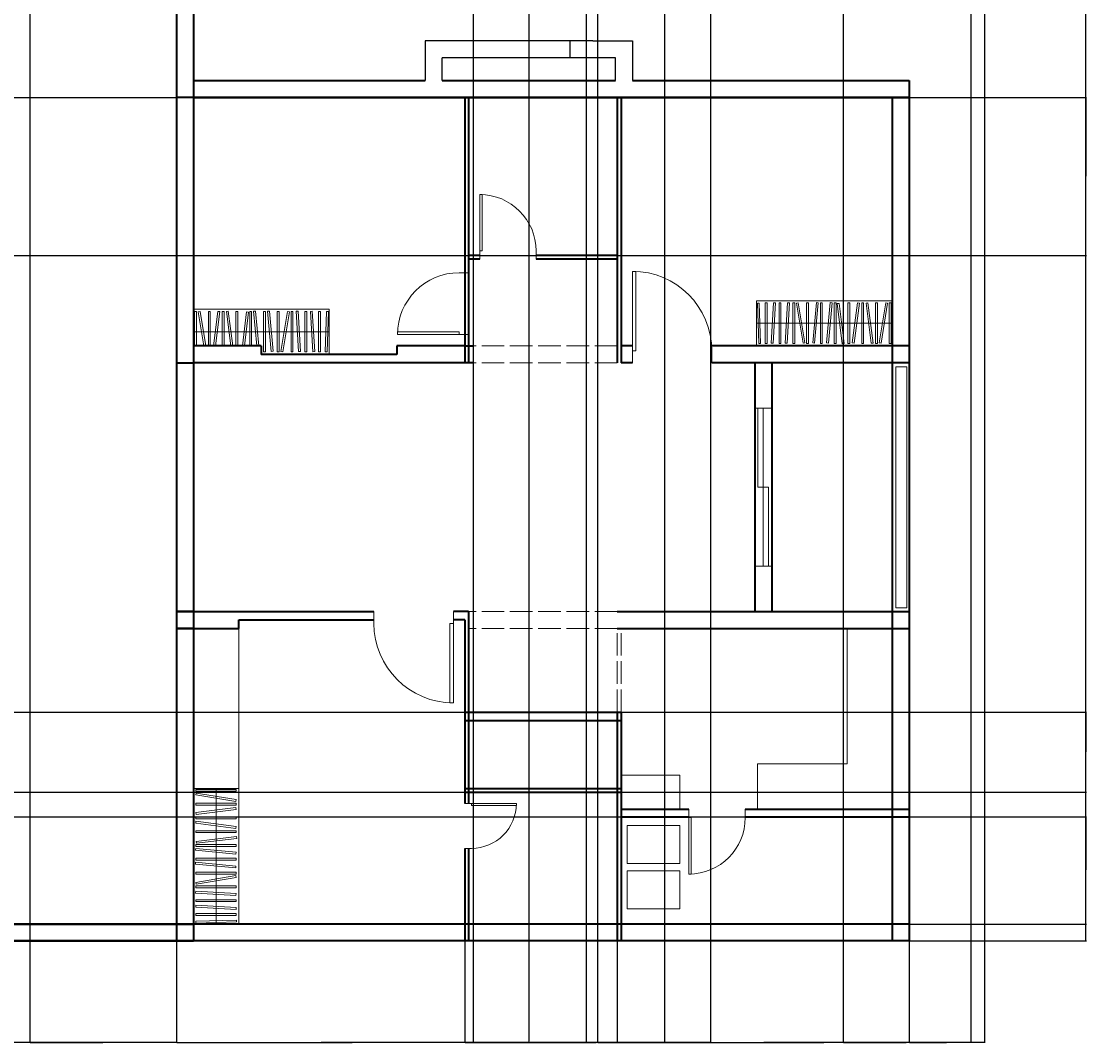
# Model space of a CAD drawing. Units: inches. Extents: x 531915 to 533151, y 849859 to 851471.
# Tile 4 of 7: x 532585 to 533151, y 850315 to 850858. Entities that reach past the tile are written whole.
import ezdxf

# ---------------------------------------------------------------- set-up
doc = ezdxf.new("R2010")
doc.units = ezdxf.units.IN
doc.linetypes.add('ACAD_ISO02W100', pattern=[15, 12, -3])
for name, color, linetype, lineweight in [('A-ANNO-DIMS', 2, 'Continuous', 18), ('A-DOOR', 3, 'Continuous', 18), ('A-FLOR-CASE', 9, 'Continuous', 18), ('A-FLOR-FIXT', 8, 'Continuous', 18), ('A-FLOR-HRAL', 4, 'Continuous', 20), ('A-FLOR-SLAB', 7, 'Continuous', 25), ('A-FURN', 8, 'Continuous', 13), ('A-NPLT-CNST', 9, 'Continuous', 9), ('A-WALL', 7, 'Continuous', 35), ('A-WALL-OVHD', 7, 'ACAD_ISO02W100', 18)]:
    doc.layers.add(name, color=color, linetype=linetype, lineweight=lineweight)
doc.styles.get("Standard").update_dxf_attribs({"font": 'arial.ttf'})
doc.dimstyles.get("Standard").update_dxf_attribs({"dimtxt": 0.18, "dimasz": 0.18, "dimexe": 0.18, "dimexo": 0.0625, "dimgap": 0.09, "dimtad": 0, "dimtih": 1, "dimtoh": 1, "dimdec": 4, "dimzin": 0, "dimdsep": 46, "dimtxsty": 'Standard', "dimcen": 0.09, "dimadec": 0, "dimazin": 0, "dimtfac": 1, "dimtdec": 4, "dimtofl": 0, "dimtmove": 0, "dimatfit": 3, "dimfxl": 1, "dimtolj": 1, "dimtzin": 0, "dimarcsym": 0})

# ---------------------------------------------------------------- blocks, each defined once
blk = doc.blocks.new('*U2')
for p, q in [((0, 0), (0, -6)), ((40, 0), (40, -6))]:
    blk.add_line(p, q)
blk.add_lwpolyline([(0, 0), (0, 40), (1.75, 40), (1.75, 0)], close=True)
blk.add_arc((0, 0), 40, 0, 90)
blk = doc.blocks.new('WARDROBE-72')
blk.add_line((12, 0), (12, 72))
for points in [[(24, 0), (24, 72), (0, 72), (0, 0)], [(1.15, 70.47), (1.15, 71.48), (22.64, 71.48), (22.64, 70.47)], [(1.21, 68.56), (1.37, 69.55), (22.58, 66.07), (22.41, 65.07)], [(1.15, 63.15), (1.15, 64.16), (22.64, 64.16), (22.64, 63.15)], [(1.15, 55.83), (1.15, 56.84), (22.64, 56.84), (22.64, 55.83)], [(1.3, 58.13), (1.17, 59.13), (22.48, 61.86), (22.61, 60.86)], [(1.11, 53.59), (1.24, 54.59), (22.54, 51.79), (22.41, 50.79)], [(1.15, 48.51), (1.15, 49.52), (22.64, 49.52), (22.64, 48.51)], [(1.55, 42.84), (1.42, 43.84), (22.76, 46.42), (22.88, 45.42)], [(1.04, 39.13), (1.13, 40.14), (22.52, 38.16), (22.43, 37.15)], [(1.15, 41.19), (1.15, 42.2), (22.64, 42.2), (22.64, 41.19)], [(1.15, 33.87), (1.15, 34.88), (22.64, 34.88), (22.64, 33.87)], [(0.98, 31.76), (1.07, 32.76), (22.47, 30.78), (22.37, 29.78)], [(1.15, 26.55), (1.15, 27.56), (22.64, 27.56), (22.64, 26.55)], [(1.38, 21.1), (1.21, 22.1), (22.4, 25.68), (22.57, 24.68)], [(1.05, 16.46), (1.11, 17.47), (22.56, 16.21), (22.5, 15.2)], [(1.15, 19.23), (1.15, 20.24), (22.64, 20.24), (22.64, 19.23)], [(1.15, 11.91), (1.15, 12.92), (22.64, 12.92), (22.64, 11.91)], [(1.11, 8.97), (1.17, 9.98), (22.62, 8.71), (22.56, 7.7)], [(1.15, 4.59), (1.15, 5.6), (22.64, 5.6), (22.64, 4.59)], [(1.25, 0.42), (1.22, 1.43), (22.7, 2.11), (22.73, 1.1)]]:
    blk.add_lwpolyline(points, close=True)
blk = doc.blocks.new('WARDROBE-72-RECESSED')
blk.add_line((0, 12), (72, 12))
for points in [[(72, 0), (72, 24), (0, 24), (0, 0), (36.16, 0)], [(37.42, 4.5), (39.13, 22.96), (40.14, 22.87), (38.44, 4.5)], [(41.19, 4.5), (41.19, 22.85), (42.2, 22.85), (42.2, 4.5)], [(48.51, 4.5), (48.51, 22.85), (49.52, 22.85), (49.52, 4.5)], [(51.17, 4.5), (53.59, 22.89), (54.59, 22.76), (52.19, 4.5)], [(55.83, 4.5), (55.83, 22.85), (56.84, 22.85), (56.84, 4.5)], [(60.46, 4.5), (58.13, 22.7), (59.13, 22.83), (61.48, 4.5)], [(63.15, 4.5), (63.15, 22.85), (64.16, 22.85), (64.16, 4.5)], [(65.55, 4.5), (68.56, 22.79), (69.55, 22.63), (66.57, 4.5)], [(70.47, 4.5), (70.47, 22.85), (71.48, 22.85), (71.48, 4.5)], [(45.01, 4.5), (42.84, 22.45), (43.84, 22.58), (46.03, 4.5)]]:
    blk.add_lwpolyline(points)
for points in [[(0.42, 22.75), (1.43, 22.78), (2.11, 1.3), (1.1, 1.27)], [(4.59, 22.85), (5.6, 22.85), (5.6, 1.36), (4.59, 1.36)], [(8.97, 22.89), (9.98, 22.83), (8.71, 1.38), (7.7, 1.44)], [(11.91, 22.85), (12.92, 22.85), (12.92, 1.36), (11.91, 1.36)], [(16.46, 22.95), (17.47, 22.89), (16.21, 1.44), (15.2, 1.5)], [(19.23, 22.85), (20.24, 22.85), (20.24, 1.36), (19.23, 1.36)], [(21.1, 22.62), (22.1, 22.79), (25.68, 1.6), (24.68, 1.43)], [(26.55, 22.85), (27.56, 22.85), (27.56, 1.36), (26.55, 1.36)], [(31.76, 23.02), (32.76, 22.93), (30.78, 1.53), (29.78, 1.63)], [(33.87, 22.85), (34.88, 22.85), (34.88, 1.36), (33.87, 1.36)]]:
    blk.add_lwpolyline(points, close=True)
blk = doc.blocks.new('BALCONY-SLIDER-84')
blk.add_line((2.88, 84), (2.88, 0))
for points in [[(2.88, 84), (5.76, 84), (5.76, 41.94), (2.88, 41.94)], [(2.88, 41.94), (0, 41.94), (0, 0), (2.88, 0)]]:
    blk.add_lwpolyline(points, close=True)
blk = doc.blocks.new('UTILITY-FIXTURES-PAIR')
for points in [[(0, 24.11), (28.12, 24.11), (28.12, 44.31), (0, 44.31)], [(0, 0), (28.12, 0), (28.12, 20.2), (0, 20.2)]]:
    blk.add_lwpolyline(points, close=True)
blk = doc.blocks.new('SERVICE-LEDGE-110')
for p, q in [((21, 21), (0, 21)), ((0, 21), (0, 0)), ((21, 21), (101, 21)), ((33, 12), (33, 21)), ((101, 21), (110, 21)), ((110, 21), (110, 0)), ((9, 0), (9, 12)), ((9, 12), (21, 12)), ((9, 12), (33, 12)), ((21, 12), (101, 12)), ((101, 0), (101, 12))]:
    blk.add_line(p, q)
blk = doc.blocks.new('COUNTER-L-RETURN')
for p, q in [((47.51, 96), (47.51, 24)), ((0, 24), (47.51, 24)), ((0, 24), (0, 0))]:
    blk.add_line(p, q)
blk = doc.blocks.new('COUNTER-END-RETURN')
for p in [(0, 18), (31.29, 0)]:
    blk.add_line(p, (31.29, 18))
blk = doc.blocks.new('*D38')
at = {"layer": 'A-ANNO-DIMS', "color": 0, "lineweight": -2, "transparency": 16777216}
for p, q in [((533096.87, 851416.87), (533150.9, 851416.87)), ((533150.72, 851416.69), (533150.72, 850893.31)), ((533150.72, 850369.55), (533150.72, 850892.94)), ((533056.87, 850369.37), (533150.9, 850369.37))]:
    blk.add_line(p, q, dxfattribs=at)
at = {"layer": 'A-ANNO-DIMS', "color": 0, "transparency": 16777216}
for points in [[(533150.69, 851416.69), (533150.75, 851416.69), (533150.72, 851416.87)], [(533150.69, 850369.55), (533150.75, 850369.55), (533150.72, 850369.37)]]:
    blk.add_solid(points, dxfattribs=at)
at = {"layer": 'Defpoints', "color": 0, "transparency": 16777216}
for p in [(533096.8, 851416.87), (533056.8, 850369.37), (533150.72, 850369.37)]:
    blk.add_point(p, dxfattribs=at)
at = {"layer": 'A-ANNO-DIMS', "color": 0, "transparency": 16777216, "insert": (533150.72, 850893.12), "char_height": 0.18, "attachment_point": 5}
blk.add_mtext('\\A1;1047.5', dxfattribs=at)
blk = doc.blocks.new('*D42')
at = {"layer": 'A-ANNO-DIMS', "color": 0, "lineweight": -2, "transparency": 16777216}
for p, q in [((532451.8, 850369.31), (532451.8, 850315.34)), ((532667.8, 850369.31), (532667.8, 850315.34)), ((532451.98, 850315.52), (532559.51, 850315.52)), ((532667.62, 850315.52), (532560.1, 850315.52))]:
    blk.add_line(p, q, dxfattribs=at)
at = {"layer": 'A-ANNO-DIMS', "color": 0, "transparency": 16777216}
for points in [[(532451.98, 850315.55), (532451.98, 850315.49), (532451.8, 850315.52)], [(532667.62, 850315.55), (532667.62, 850315.49), (532667.8, 850315.52)]]:
    blk.add_solid(points, dxfattribs=at)
at = {"layer": 'Defpoints', "color": 0, "transparency": 16777216}
for p in [(532451.8, 850369.37), (532667.8, 850369.37), (532667.8, 850315.52)]:
    blk.add_point(p, dxfattribs=at)
at = {"layer": 'A-ANNO-DIMS', "color": 0, "transparency": 16777216, "insert": (532559.8, 850315.52), "char_height": 0.18, "attachment_point": 5}
blk.add_mtext('\\A1;216', dxfattribs=at)
blk = doc.blocks.new('*D43')
at = {"layer": 'A-ANNO-DIMS', "color": 0, "lineweight": -2, "transparency": 16777216}
for p, q in [((532667.8, 850369.31), (532667.8, 850315.34)), ((532820.8, 850369.31), (532820.8, 850315.34)), ((532667.98, 850315.52), (532744.02, 850315.52)), ((532820.62, 850315.52), (532744.59, 850315.52))]:
    blk.add_line(p, q, dxfattribs=at)
at = {"layer": 'A-ANNO-DIMS', "color": 0, "transparency": 16777216}
for points in [[(532667.98, 850315.55), (532667.98, 850315.49), (532667.8, 850315.52)], [(532820.62, 850315.55), (532820.62, 850315.49), (532820.8, 850315.52)]]:
    blk.add_solid(points, dxfattribs=at)
at = {"layer": 'Defpoints', "color": 0, "transparency": 16777216}
for p in [(532667.8, 850369.37), (532820.8, 850369.37), (532820.8, 850315.52)]:
    blk.add_point(p, dxfattribs=at)
at = {"layer": 'A-ANNO-DIMS', "color": 0, "transparency": 16777216, "insert": (532744.3, 850315.52), "char_height": 0.18, "attachment_point": 5}
blk.add_mtext('\\A1;153', dxfattribs=at)
blk = doc.blocks.new('*D44')
at = {"layer": 'A-ANNO-DIMS', "color": 0, "lineweight": -2, "transparency": 16777216}
for p, q in [((532820.8, 850369.31), (532820.8, 850315.34)), ((532901.8, 850369.31), (532901.8, 850315.34)), ((532820.98, 850315.52), (532861.1, 850315.52)), ((532901.62, 850315.52), (532861.51, 850315.52))]:
    blk.add_line(p, q, dxfattribs=at)
at = {"layer": 'A-ANNO-DIMS', "color": 0, "transparency": 16777216}
for points in [[(532820.98, 850315.55), (532820.98, 850315.49), (532820.8, 850315.52)], [(532901.62, 850315.55), (532901.62, 850315.49), (532901.8, 850315.52)]]:
    blk.add_solid(points, dxfattribs=at)
at = {"layer": 'Defpoints', "color": 0, "transparency": 16777216}
for p in [(532820.8, 850369.37), (532901.8, 850369.37), (532901.8, 850315.52)]:
    blk.add_point(p, dxfattribs=at)
at = {"layer": 'A-ANNO-DIMS', "color": 0, "transparency": 16777216, "insert": (532861.3, 850315.52), "char_height": 0.18, "attachment_point": 5}
blk.add_mtext('\\A1;81', dxfattribs=at)
blk = doc.blocks.new('*D45')
at = {"layer": 'A-ANNO-DIMS', "color": 0, "lineweight": -2, "transparency": 16777216}
for p, q in [((532901.8, 850369.31), (532901.8, 850315.34)), ((533056.8, 850369.31), (533056.8, 850315.34)), ((532901.98, 850315.52), (532979.02, 850315.52)), ((533056.62, 850315.52), (532979.59, 850315.52))]:
    blk.add_line(p, q, dxfattribs=at)
at = {"layer": 'A-ANNO-DIMS', "color": 0, "transparency": 16777216}
for points in [[(532901.98, 850315.55), (532901.98, 850315.49), (532901.8, 850315.52)], [(533056.62, 850315.55), (533056.62, 850315.49), (533056.8, 850315.52)]]:
    blk.add_solid(points, dxfattribs=at)
at = {"layer": 'Defpoints', "color": 0, "transparency": 16777216}
for p in [(532901.8, 850369.37), (533056.8, 850369.37), (533056.8, 850315.52)]:
    blk.add_point(p, dxfattribs=at)
at = {"layer": 'A-ANNO-DIMS', "color": 0, "transparency": 16777216, "insert": (532979.3, 850315.52), "char_height": 0.18, "attachment_point": 5}
blk.add_mtext('\\A1;155', dxfattribs=at)
blk = doc.blocks.new('*D47')
at = {"layer": 'A-ANNO-DIMS', "color": 0, "lineweight": -2, "transparency": 16777216}
for p, q in [((533096.8, 850946.31), (533096.8, 850315.34)), ((533056.8, 850826.31), (533056.8, 850315.34)), ((533056.98, 850315.52), (533076.58, 850315.52)), ((533096.62, 850315.52), (533077.03, 850315.52))]:
    blk.add_line(p, q, dxfattribs=at)
at = {"layer": 'A-ANNO-DIMS', "color": 0, "transparency": 16777216}
for points in [[(533056.98, 850315.55), (533056.98, 850315.49), (533056.8, 850315.52)], [(533096.62, 850315.55), (533096.62, 850315.49), (533096.8, 850315.52)]]:
    blk.add_solid(points, dxfattribs=at)
at = {"layer": 'Defpoints', "color": 0, "transparency": 16777216}
for p in [(533096.8, 850946.37), (533056.8, 850826.37), (533056.8, 850315.52)]:
    blk.add_point(p, dxfattribs=at)
at = {"layer": 'A-ANNO-DIMS', "color": 0, "transparency": 16777216, "insert": (533076.8, 850315.52), "char_height": 0.18, "attachment_point": 5}
blk.add_mtext('\\A1;40', dxfattribs=at)
blk = doc.blocks.new('*D49')
at = {"layer": 'A-ANNO-DIMS', "color": 0, "lineweight": -2, "transparency": 16777216}
for p, q in [((532825.3, 851312.76), (532825.3, 850315.34)), ((532885.3, 851312.76), (532885.3, 850315.34)), ((532825.48, 850315.52), (532855.09, 850315.52)), ((532885.12, 850315.52), (532855.52, 850315.52))]:
    blk.add_line(p, q, dxfattribs=at)
at = {"layer": 'A-ANNO-DIMS', "color": 0, "transparency": 16777216}
for points in [[(532825.48, 850315.55), (532825.48, 850315.49), (532825.3, 850315.52)], [(532885.12, 850315.55), (532885.12, 850315.49), (532885.3, 850315.52)]]:
    blk.add_solid(points, dxfattribs=at)
at = {"layer": 'Defpoints', "color": 0, "transparency": 16777216}
for p in [(532825.3, 851312.82), (532885.3, 851312.82), (532885.3, 850315.52)]:
    blk.add_point(p, dxfattribs=at)
at = {"layer": 'A-ANNO-DIMS', "color": 0, "transparency": 16777216, "insert": (532855.3, 850315.52), "char_height": 0.18, "attachment_point": 5}
blk.add_mtext('\\A1;60', dxfattribs=at)
blk = doc.blocks.new('*D50')
at = {"layer": 'A-ANNO-DIMS', "color": 0, "lineweight": -2, "transparency": 16777216}
for p, q in [((532891.3, 851312.76), (532891.3, 850315.34)), ((532951.3, 851312.76), (532951.3, 850315.34)), ((532891.48, 850315.52), (532921.09, 850315.52)), ((532951.12, 850315.52), (532921.52, 850315.52))]:
    blk.add_line(p, q, dxfattribs=at)
at = {"layer": 'A-ANNO-DIMS', "color": 0, "transparency": 16777216}
for points in [[(532891.48, 850315.55), (532891.48, 850315.49), (532891.3, 850315.52)], [(532951.12, 850315.55), (532951.12, 850315.49), (532951.3, 850315.52)]]:
    blk.add_solid(points, dxfattribs=at)
at = {"layer": 'Defpoints', "color": 0, "transparency": 16777216}
for p in [(532891.3, 851312.82), (532951.3, 851312.82), (532951.3, 850315.52)]:
    blk.add_point(p, dxfattribs=at)
at = {"layer": 'A-ANNO-DIMS', "color": 0, "transparency": 16777216, "insert": (532921.3, 850315.52), "char_height": 0.18, "attachment_point": 5}
blk.add_mtext('\\A1;60', dxfattribs=at)
blk = doc.blocks.new('*D55')
at = {"layer": 'A-ANNO-DIMS', "color": 0, "lineweight": -2, "transparency": 16777216}
for p, q in [((532667.8, 850946.31), (532667.8, 850315.34)), ((532854.8, 850946.31), (532854.8, 850315.34)), ((532667.98, 850315.52), (532761.02, 850315.52)), ((532854.62, 850315.52), (532761.59, 850315.52))]:
    blk.add_line(p, q, dxfattribs=at)
at = {"layer": 'A-ANNO-DIMS', "color": 0, "transparency": 16777216}
for points in [[(532667.98, 850315.55), (532667.98, 850315.49), (532667.8, 850315.52)], [(532854.62, 850315.55), (532854.62, 850315.49), (532854.8, 850315.52)]]:
    blk.add_solid(points, dxfattribs=at)
at = {"layer": 'Defpoints', "color": 0, "transparency": 16777216}
for p in [(532667.8, 850946.37), (532854.8, 850946.37), (532854.8, 850315.52)]:
    blk.add_point(p, dxfattribs=at)
at = {"layer": 'A-ANNO-DIMS', "color": 0, "transparency": 16777216, "insert": (532761.3, 850315.52), "char_height": 0.18, "attachment_point": 5}
blk.add_mtext('\\A1;187', dxfattribs=at)
blk = doc.blocks.new('*D56')
at = {"layer": 'A-ANNO-DIMS', "color": 0, "lineweight": -2, "transparency": 16777216}
for p, q in [((532854.8, 850946.31), (532854.8, 850315.34)), ((532926.8, 850946.31), (532926.8, 850315.34)), ((532854.98, 850315.52), (532890.59, 850315.52)), ((532926.62, 850315.52), (532891.02, 850315.52))]:
    blk.add_line(p, q, dxfattribs=at)
at = {"layer": 'A-ANNO-DIMS', "color": 0, "transparency": 16777216}
for points in [[(532854.98, 850315.55), (532854.98, 850315.49), (532854.8, 850315.52)], [(532926.62, 850315.55), (532926.62, 850315.49), (532926.8, 850315.52)]]:
    blk.add_solid(points, dxfattribs=at)
at = {"layer": 'Defpoints', "color": 0, "transparency": 16777216}
for p in [(532854.8, 850946.37), (532926.8, 850946.37), (532926.8, 850315.52)]:
    blk.add_point(p, dxfattribs=at)
at = {"layer": 'A-ANNO-DIMS', "color": 0, "transparency": 16777216, "insert": (532890.8, 850315.52), "char_height": 0.18, "attachment_point": 5}
blk.add_mtext('\\A1;72', dxfattribs=at)
blk = doc.blocks.new('*D57')
at = {"layer": 'A-ANNO-DIMS', "color": 0, "lineweight": -2, "transparency": 16777216}
for p, q in [((532926.8, 850946.31), (532926.8, 850315.34)), ((533096.8, 850946.31), (533096.8, 850315.34)), ((532926.98, 850315.52), (533011.52, 850315.52)), ((533096.62, 850315.52), (533012.08, 850315.52))]:
    blk.add_line(p, q, dxfattribs=at)
at = {"layer": 'A-ANNO-DIMS', "color": 0, "transparency": 16777216}
for points in [[(532926.98, 850315.55), (532926.98, 850315.49), (532926.8, 850315.52)], [(533096.62, 850315.55), (533096.62, 850315.49), (533096.8, 850315.52)]]:
    blk.add_solid(points, dxfattribs=at)
at = {"layer": 'Defpoints', "color": 0, "transparency": 16777216}
for p in [(532926.8, 850946.37), (533096.8, 850946.37), (533096.8, 850315.52)]:
    blk.add_point(p, dxfattribs=at)
at = {"layer": 'A-ANNO-DIMS', "color": 0, "transparency": 16777216, "insert": (533011.8, 850315.52), "char_height": 0.18, "attachment_point": 5}
blk.add_mtext('\\A1;170', dxfattribs=at)
blk = doc.blocks.new('*D58')
at = {"layer": 'A-ANNO-DIMS', "color": 0, "lineweight": -2, "transparency": 16777216}
for p, q in [((533021.8, 851259.31), (533021.8, 850315.34)), ((533089.48, 851257.99), (533089.48, 850315.34)), ((533021.98, 850315.52), (533055.25, 850315.52)), ((533089.3, 850315.52), (533056.04, 850315.52))]:
    blk.add_line(p, q, dxfattribs=at)
at = {"layer": 'A-ANNO-DIMS', "color": 0, "transparency": 16777216}
for points in [[(533021.98, 850315.55), (533021.98, 850315.49), (533021.8, 850315.52)], [(533089.3, 850315.55), (533089.3, 850315.49), (533089.48, 850315.52)]]:
    blk.add_solid(points, dxfattribs=at)
at = {"layer": 'Defpoints', "color": 0, "transparency": 16777216}
for p in [(533021.8, 851259.37), (533089.48, 851258.05), (533089.48, 850315.52)]:
    blk.add_point(p, dxfattribs=at)
at = {"layer": 'A-ANNO-DIMS', "color": 0, "transparency": 16777216, "insert": (533055.64, 850315.52), "char_height": 0.18, "attachment_point": 5}
blk.add_mtext('\\A1;67.67', dxfattribs=at)
blk = doc.blocks.new('*D67')
at = {"layer": 'A-ANNO-DIMS', "color": 0, "lineweight": -2, "transparency": 16777216}
for p, q in [((532451.87, 850435.37), (533150.9, 850435.37)), ((533150.72, 850435.19), (533150.72, 850407.06)), ((533150.72, 850378.55), (533150.72, 850406.69)), ((532442.87, 850378.37), (533150.9, 850378.37))]:
    blk.add_line(p, q, dxfattribs=at)
at = {"layer": 'A-ANNO-DIMS', "color": 0, "transparency": 16777216}
for points in [[(533150.69, 850435.19), (533150.75, 850435.19), (533150.72, 850435.37)], [(533150.69, 850378.55), (533150.75, 850378.55), (533150.72, 850378.37)]]:
    blk.add_solid(points, dxfattribs=at)
at = {"layer": 'Defpoints', "color": 0, "transparency": 16777216}
for p in [(532451.8, 850435.37), (532442.8, 850378.37), (533150.72, 850378.37)]:
    blk.add_point(p, dxfattribs=at)
at = {"layer": 'A-ANNO-DIMS', "color": 0, "transparency": 16777216, "insert": (533150.72, 850406.87), "char_height": 0.18, "attachment_point": 5}
blk.add_mtext('\\A1;57', dxfattribs=at)
blk = doc.blocks.new('*D71')
at = {"layer": 'A-ANNO-DIMS', "color": 0, "lineweight": -2, "transparency": 16777216}
for p, q in [((532589.8, 850931.17), (532589.8, 850315.34)), ((532667.8, 850931.17), (532667.8, 850315.34)), ((532589.98, 850315.52), (532628.59, 850315.52)), ((532667.62, 850315.52), (532629.02, 850315.52))]:
    blk.add_line(p, q, dxfattribs=at)
at = {"layer": 'A-ANNO-DIMS', "color": 0, "transparency": 16777216}
for points in [[(532589.98, 850315.55), (532589.98, 850315.49), (532589.8, 850315.52)], [(532667.62, 850315.55), (532667.62, 850315.49), (532667.8, 850315.52)]]:
    blk.add_solid(points, dxfattribs=at)
at = {"layer": 'Defpoints', "color": 0, "transparency": 16777216}
for p in [(532589.8, 850931.23), (532667.8, 850931.23), (532667.8, 850315.52)]:
    blk.add_point(p, dxfattribs=at)
at = {"layer": 'A-ANNO-DIMS', "color": 0, "transparency": 16777216, "insert": (532628.8, 850315.52), "char_height": 0.18, "attachment_point": 5}
blk.add_mtext('\\A1;78', dxfattribs=at)
blk = doc.blocks.new('*D77')
at = {"layer": 'A-ANNO-DIMS', "color": 0, "lineweight": -2, "transparency": 16777216}
for p, q in [((532215.87, 850817.37), (533150.9, 850817.37)), ((533150.72, 850817.19), (533150.72, 850775.56)), ((533150.72, 850733.55), (533150.72, 850775.19)), ((532217.87, 850733.37), (533150.9, 850733.37))]:
    blk.add_line(p, q, dxfattribs=at)
at = {"layer": 'A-ANNO-DIMS', "color": 0, "transparency": 16777216}
for points in [[(533150.69, 850817.19), (533150.75, 850817.19), (533150.72, 850817.37)], [(533150.69, 850733.55), (533150.75, 850733.55), (533150.72, 850733.37)]]:
    blk.add_solid(points, dxfattribs=at)
at = {"layer": 'Defpoints', "color": 0, "transparency": 16777216}
for p in [(532215.8, 850817.37), (532217.8, 850733.37), (533150.72, 850733.37)]:
    blk.add_point(p, dxfattribs=at)
at = {"layer": 'A-ANNO-DIMS', "color": 0, "transparency": 16777216, "insert": (533150.72, 850775.37), "char_height": 0.18, "attachment_point": 5}
blk.add_mtext('\\A1;84', dxfattribs=at)
blk = doc.blocks.new('*D84')
at = {"layer": 'A-ANNO-DIMS', "color": 0, "lineweight": -2, "transparency": 16777216}
for p, q in [((532215.87, 850490.87), (533150.9, 850490.87)), ((533150.72, 850490.69), (533150.72, 850469.81)), ((533150.72, 850448.55), (533150.72, 850469.44)), ((532215.87, 850448.37), (533150.9, 850448.37))]:
    blk.add_line(p, q, dxfattribs=at)
at = {"layer": 'A-ANNO-DIMS', "color": 0, "transparency": 16777216}
for points in [[(533150.69, 850490.69), (533150.75, 850490.69), (533150.72, 850490.87)], [(533150.69, 850448.55), (533150.75, 850448.55), (533150.72, 850448.37)]]:
    blk.add_solid(points, dxfattribs=at)
at = {"layer": 'Defpoints', "color": 0, "transparency": 16777216}
for p in [(532215.8, 850490.87), (532215.8, 850448.37), (533150.72, 850448.37)]:
    blk.add_point(p, dxfattribs=at)
at = {"layer": 'A-ANNO-DIMS', "color": 0, "transparency": 16777216, "insert": (533150.72, 850469.62), "char_height": 0.18, "attachment_point": 5}
blk.add_mtext('\\A1;42.5', dxfattribs=at)

msp = doc.modelspace()

# ---------------------------------------------------------------- linework, layer by layer
at = {"layer": 'A-DOOR'}
for p, q in [((532983.8048, 850652.374), (532974.8048, 850652.374)), ((532983.8048, 850568.374), (532974.8048, 850568.374))]:
    msp.add_line(p, q, dxfattribs=at)
at = {"layer": 'A-FLOR-HRAL'}
msp.add_lwpolyline([(533055.5138, 850674.239), (533049.7847, 850674.239), (533049.7847, 850546.2421), (533055.5138, 850546.2421)], close=True, dxfattribs=at)
at = {"layer": 'A-FURN'}
msp.add_line((532700.8048, 850450.374), (532700.8048, 850535.374), dxfattribs=at)
at = {"layer": 'A-NPLT-CNST'}
for p in [(532081.8048, 850249.374), (532081.8048, 850240.374), (532306.3048, 850120.374), (532081.8048, 850111.374), (532081.8048, 849991.374), (532081.8048, 849982.374), (532081.8048, 849859.374)]:
    msp.add_ray(p, (1, 0), dxfattribs=at)
at = {"layer": 'A-WALL'}
for p, q in [((532667.8048, 851211.374), (532667.8048, 850369.374)), ((532676.8048, 850946.374), (532676.8048, 850369.374)), ((532667.8048, 850931.2344), (532667.8048, 850369.374)), ((532676.8048, 850931.2344), (532676.8048, 850369.374)), ((532676.8048, 850826.374), (532799.8048, 850826.374)), ((532808.8048, 850826.374), (532900.8048, 850826.374)), ((532909.8048, 850826.374), (533056.8048, 850826.374)), ((533056.8048, 850826.374), (533056.8048, 850369.374)), ((533056.8048, 850817.374), (532667.8048, 850817.374)), ((532676.8048, 850817.374), (533056.8048, 850817.374)), ((532820.8048, 850817.374), (532820.8048, 850724.227)), ((532820.8048, 850817.374), (532820.8048, 850676.374)), ((532822.8048, 850817.374), (532822.8048, 850724.227)), ((532901.8048, 850817.374), (532822.8048, 850817.374)), ((532822.8048, 850817.374), (532822.8048, 850676.374)), ((532901.8048, 850817.374), (532901.8048, 850676.374)), ((532903.8048, 850817.374), (532903.8048, 850676.374)), ((533047.8048, 850817.374), (533047.8048, 850369.374)), ((532828.8048, 850733.374), (532822.8048, 850733.374)), ((532901.8048, 850733.374), (532858.6883, 850733.374)), ((532828.8048, 850731.374), (532822.8048, 850731.374)), ((532901.8048, 850731.374), (532858.6883, 850731.374)), ((532820.8048, 850691.374), (532820.8048, 850676.374)), ((532822.8048, 850691.374), (532822.8048, 850676.374)), ((532712.6447, 850685.374), (532676.8048, 850685.374)), ((532712.6447, 850685.374), (532712.6447, 850680.874)), ((532820.4846, 850685.374), (532784.6447, 850685.374)), ((532820.4846, 850685.374), (532784.6447, 850685.374)), ((532820.4846, 850685.374), (532784.6447, 850685.374)), ((532784.6447, 850685.374), (532784.6447, 850680.874)), ((532820.4846, 850685.374), (532825.3048, 850685.374)), ((532909.8048, 850685.374), (532903.8048, 850685.374)), ((533056.8048, 850685.374), (532951.9726, 850685.374)), ((532667.8048, 850676.374), (532676.8048, 850676.374)), ((532820.8048, 850676.374), (532676.8048, 850676.374)), ((532825.3048, 850676.374), (532676.8048, 850676.374)), ((532784.6447, 850680.874), (532712.6447, 850680.874)), ((532909.8048, 850676.374), (532903.8048, 850676.374)), ((533056.8048, 850676.374), (532952.0565, 850676.374)), ((532974.8048, 850676.374), (532974.8048, 850544.374)), ((532983.8048, 850676.374), (532983.8048, 850544.374)), ((532676.8048, 850544.374), (532667.8048, 850544.374)), ((532667.8048, 850544.374), (532772.553, 850544.374)), ((532667.8048, 850544.374), (532676.8048, 850544.374)), ((532820.8048, 850544.374), (532814.8048, 850544.374)), ((532822.8048, 850544.374), (532820.8048, 850544.374)), ((532822.8048, 850544.374), (532822.8048, 850442.374)), ((532901.8048, 850544.374), (533056.8048, 850544.374)), ((532676.8048, 850535.374), (532667.8048, 850535.374)), ((532667.8048, 850535.374), (532700.8048, 850535.374)), ((532667.8048, 850535.374), (532676.8048, 850535.374)), ((532676.8048, 850535.374), (532700.8048, 850535.374)), ((532700.8048, 850535.374), (532700.8048, 850539.874)), ((532700.8048, 850539.874), (532772.553, 850539.874)), ((532820.8048, 850539.874), (532814.8048, 850539.874)), ((532820.8048, 850539.874), (532820.8048, 850442.374)), ((532901.8048, 850535.374), (533056.8048, 850535.374)), ((532820.8048, 850490.874), (532903.8048, 850490.874)), ((532901.8048, 850490.874), (532901.8048, 850369.374)), ((532903.8048, 850490.874), (532903.8048, 850369.374)), ((532820.8048, 850486.374), (532903.8048, 850486.374)), ((532820.8048, 850450.374), (532903.8048, 850450.374)), ((532820.8048, 850448.374), (532903.8048, 850448.374)), ((532903.8048, 850439.374), (532939.8048, 850439.374)), ((532969.7592, 850439.374), (533056.8048, 850439.374)), ((532903.8048, 850435.374), (532939.8048, 850435.374)), ((532969.7592, 850435.374), (533056.8048, 850435.374)), ((532820.8048, 850418.5523), (532820.8048, 850369.374)), ((532822.8048, 850418.5523), (532822.8048, 850369.374)), ((532062.8048, 850378.374), (532676.8048, 850378.374)), ((533056.8048, 850378.374), (532442.8048, 850378.374)), ((532062.8048, 850369.374), (532676.8048, 850369.374)), ((533056.8048, 850369.374), (532442.8048, 850369.374))]:
    msp.add_line(p, q, dxfattribs=at)
at = {"layer": 'A-WALL-OVHD'}
for p, q in [((532901.8048, 850685.374), (532822.8048, 850685.374)), ((532901.8048, 850676.374), (532822.8048, 850676.374)), ((532901.8048, 850544.374), (532822.8048, 850544.374)), ((532901.8048, 850535.374), (532822.8048, 850535.374)), ((532901.8048, 850490.874), (532901.8048, 850535.374)), ((532903.8048, 850490.874), (532903.8048, 850535.374))]:
    msp.add_line(p, q, dxfattribs=at)

# ---------------------------------------------------------------- block references
at = {"layer": 'A-DOOR'}
for p, xscale, yscale, zscale in [((532828.8048, 850735.8565), 0.7470890379753774, 0.7470890379753774, 0.7470890379753774), ((532909.8048, 850682.7117), 1.056294156906435, 1.056294156906435, 1.056294156906435)]:
    msp.add_blockref('*U2', p, dxfattribs=dict(at, xscale=xscale, yscale=yscale, zscale=zscale))
for p, xscale, yscale, zscale, rotation in [((532817.9128, 850691.374), 0.8213266256042635, 0.8213266256042635, 0.8213266256042635, 90.00000000000003), ((532814.8048, 850538.0362), 1.056294156906435, 1.056294156906435, 1.056294156906435, 180), ((532824.378, 850442.374), 0.5955413682082586, 0.5955413682082586, 0.5955413682082586, 270), ((532939.8048, 850434.8808), -0.7488601199280389, 0.7488601199280389, 0.7488601199280389, 180)]:
    msp.add_blockref('*U2', p, dxfattribs=dict(at, xscale=xscale, yscale=yscale, zscale=zscale, rotation=rotation))
at = {"layer": 'A-DOOR', "extrusion": (0, 0, -1), "zscale": -1}
msp.add_blockref('BALCONY-SLIDER-84', (-532982.142, 850568.374), dxfattribs=at)
at = {"layer": 'A-FLOR-CASE'}
for name, p in [('COUNTER-L-RETURN', (532976.2933, 850439.374)), ('COUNTER-END-RETURN', (532903.8048, 850439.374))]:
    msp.add_blockref(name, p, dxfattribs=at)
at = {"layer": 'A-FLOR-FIXT'}
msp.add_blockref('UTILITY-FIXTURES-PAIR', (532906.9813, 850386.385), dxfattribs=at)
at = {"layer": 'A-FLOR-SLAB', "extrusion": (0, 0, -1), "zscale": -1}
msp.add_blockref('SERVICE-LEDGE-110', (-532909.8048, 850826.374), dxfattribs=at)
at = {"layer": 'A-FURN', "extrusion": (0, 0, -1), "zscale": -1}
msp.add_blockref('WARDROBE-72-RECESSED', (-532748.8048, 850680.874), dxfattribs=at)
at = {"layer": 'A-FURN', "rotation": 269.9999999995917}
msp.add_blockref('WARDROBE-72', (532975.8048, 850709.374), dxfattribs=at)
at = {"layer": 'A-FURN'}
msp.add_blockref('WARDROBE-72', (532676.8048, 850378.374), dxfattribs=at)

# ---------------------------------------------------------------- dimensions: what is measured, and where the dimension line sits
at = {"layer": 'A-ANNO-DIMS'}
for base, p1, p2, override, picture, middle in [((533150.7156, 850369.374), (533096.8048, 851416.874), (533056.8048, 850369.374), {"dimdec": 1, "dimlfac": 1, "dimrnd": 0, "dimzin": 0, "dimdsep": 46, "dimlunit": 2}, '*D38', (533150.7156, 850893.124)), ((533150.7156, 850733.374), (532215.8048, 850817.374), (532217.8048, 850733.374), {"dimdec": 0, "dimlfac": 1, "dimrnd": 0, "dimzin": 0, "dimdsep": 46, "dimlunit": 2}, '*D77', (533150.7156, 850775.374)), ((533150.7156, 850448.374), (532215.8048, 850490.874), (532215.8048, 850448.374), {"dimdec": 1, "dimlfac": 1, "dimrnd": 0, "dimzin": 0, "dimdsep": 46, "dimlunit": 2}, '*D84', (533150.7156, 850469.624)), ((533150.7156, 850378.374), (532451.8048, 850435.374), (532442.8048, 850378.374), {"dimdec": 0, "dimlfac": 1, "dimrnd": 0, "dimzin": 0, "dimdsep": 46, "dimlunit": 2}, '*D67', (533150.7156, 850406.874))]:
    dim = msp.add_linear_dim(base=base, p1=p1, p2=p2, angle=90, dimstyle='Standard', override=override, dxfattribs=at)
    dim.commit()
    dim.dimension.update_dxf_attribs({"geometry": picture, "text_midpoint": middle})
for base, p1, p2, override, picture, middle in [((532885.3048, 850315.524), (532825.3048, 851312.8243), (532885.3048, 851312.8243), {"dimdec": 0, "dimlfac": 1, "dimrnd": 0, "dimzin": 0, "dimdsep": 46, "dimlunit": 2}, '*D49', (532855.3048, 850315.524)), ((532951.3048, 850315.524), (532891.3048, 851312.8243), (532951.3048, 851312.8243), {"dimdec": 0, "dimlfac": 1, "dimrnd": 0, "dimzin": 0, "dimdsep": 46, "dimlunit": 2}, '*D50', (532921.3048, 850315.524)), ((533089.477, 850315.524), (533021.8048, 851259.374), (533089.477, 851258.0527), {"dimdec": 2, "dimlfac": 1, "dimrnd": 0, "dimzin": 0, "dimdsep": 46, "dimlunit": 2}, '*D58', (533055.6409, 850315.524)), ((532854.8048, 850315.524), (532667.8048, 850946.374), (532854.8048, 850946.374), {"dimdec": 0, "dimlfac": 1, "dimrnd": 0, "dimzin": 0, "dimdsep": 46, "dimlunit": 2}, '*D55', (532761.3048, 850315.524)), ((532926.8048, 850315.524), (532854.8048, 850946.374), (532926.8048, 850946.374), {"dimdec": 0, "dimlfac": 1, "dimrnd": 0, "dimzin": 0, "dimdsep": 46, "dimlunit": 2}, '*D56', (532890.8048, 850315.524)), ((533096.8048, 850315.524), (532926.8048, 850946.374), (533096.8048, 850946.374), {"dimdec": 0, "dimlfac": 1, "dimrnd": 0, "dimzin": 0, "dimdsep": 46, "dimlunit": 2}, '*D57', (533011.8048, 850315.524)), ((533056.8048, 850315.524), (533096.8048, 850946.374), (533056.8048, 850826.374), {"dimdec": 0, "dimlfac": 1, "dimrnd": 0, "dimzin": 0, "dimdsep": 46, "dimlunit": 2}, '*D47', (533076.8048, 850315.524)), ((532667.8048, 850315.524), (532589.8048, 850931.2344), (532667.8048, 850931.2344), {"dimdec": 0, "dimlfac": 1, "dimrnd": 0, "dimzin": 0, "dimdsep": 46, "dimlunit": 2}, '*D71', (532628.8048, 850315.524)), ((532667.8048, 850315.524), (532451.8048, 850369.374), (532667.8048, 850369.374), {"dimdec": 0, "dimlfac": 1, "dimrnd": 0, "dimzin": 0, "dimdsep": 46, "dimlunit": 2}, '*D42', (532559.8048, 850315.524)), ((532820.8048, 850315.524), (532667.8048, 850369.374), (532820.8048, 850369.374), {"dimdec": 0, "dimlfac": 1, "dimrnd": 0, "dimzin": 0, "dimdsep": 46, "dimlunit": 2}, '*D43', (532744.3048, 850315.524)), ((532901.8048, 850315.524), (532820.8048, 850369.374), (532901.8048, 850369.374), {"dimdec": 0, "dimlfac": 1, "dimrnd": 0, "dimzin": 0, "dimdsep": 46, "dimlunit": 2}, '*D44', (532861.3048, 850315.524)), ((533056.8048, 850315.524), (532901.8048, 850369.374), (533056.8048, 850369.374), {"dimdec": 0, "dimlfac": 1, "dimrnd": 0, "dimzin": 0, "dimdsep": 46, "dimlunit": 2}, '*D45', (532979.3048, 850315.524))]:
    dim = msp.add_linear_dim(base=base, p1=p1, p2=p2, dimstyle='Standard', override=override, dxfattribs=at)
    dim.commit()
    dim.dimension.update_dxf_attribs({"geometry": picture, "text_midpoint": middle})

doc.saveas('drawing.dxf')
